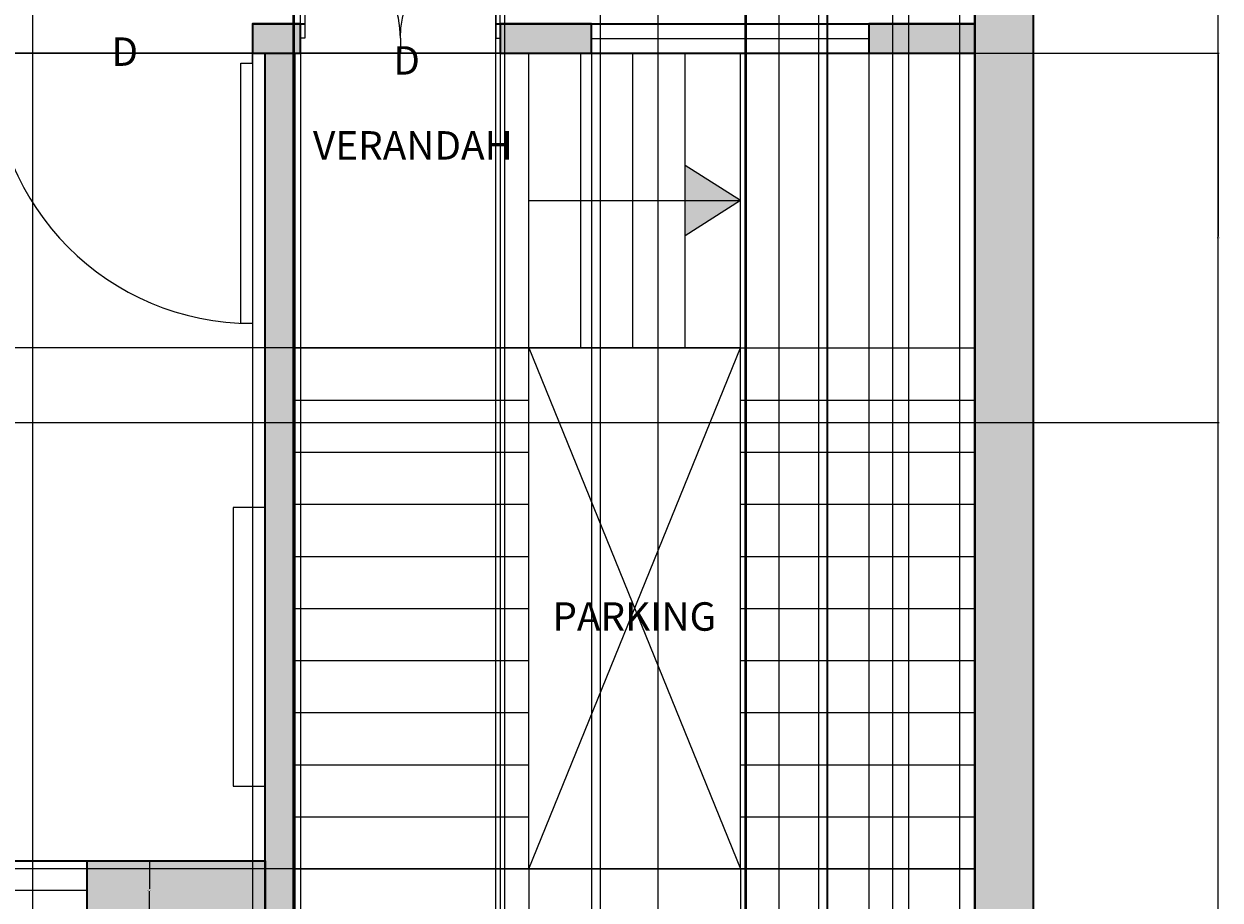
# Model space of a CAD drawing. Units: inches. Extents: x 2035 to 2384, y 1427 to 2020.
# Tile 3 of 7: x 2200 to 2383, y 1551 to 1685. Entities that reach past the tile are written whole.
import ezdxf

# ---------------------------------------------------------------- set-up
doc = ezdxf.new("R2010")
doc.units = ezdxf.units.IN
for name, color, linetype, lineweight in [('A-ANNO-DIMS', 2, 'Continuous', 18), ('A-ANNO-IDEN', 201, 'Continuous', 18), ('A-ANNO-SYMB', 201, 'Continuous', 18), ('A-AREA-IDEN', 201, 'Continuous', 18), ('A-FLOR-STRS', 8, 'Continuous', 18), ('A-WALL-PATT', 140, 'Continuous', 13), ('C-PROP', 7, 'Continuous', 25), ('DOOR', 52, 'Continuous', 25), ('FUR', 71, 'Continuous', 18), ('WALL', 140, 'Continuous', 35), ('WIN', 230, 'Continuous', 18)]:
    doc.layers.add(name, color=color, linetype=linetype, lineweight=lineweight)
doc.styles.get("Standard").update_dxf_attribs({"font": 'arial.ttf'})
doc.dimstyles.get("Standard").update_dxf_attribs({"dimtxt": 0.18, "dimasz": 0.18, "dimexe": 0.18, "dimexo": 0.0625, "dimgap": 0.09, "dimtad": 0, "dimtih": 1, "dimtoh": 1, "dimdec": 4, "dimzin": 0, "dimdsep": 46, "dimtxsty": 'Standard', "dimcen": 0.09, "dimadec": 0, "dimazin": 0, "dimtfac": 1, "dimtdec": 4, "dimtofl": 0, "dimtmove": 0, "dimatfit": 3, "dimfxl": 1, "dimtolj": 1, "dimtzin": 0, "dimarcsym": 0})

# ---------------------------------------------------------------- blocks, each defined once
blk = doc.blocks.new('*U2')
for p, q in [((0, 0), (0, -6)), ((40, 0), (40, -6))]:
    blk.add_line(p, q)
blk.add_lwpolyline([(0, 0), (0, 40), (1.75, 40), (1.75, 0)], close=True)
blk.add_arc((0, 0), 40, 0, 90)
blk = doc.blocks.new('WIN-BEDROOM')
blk.add_line((0, 4.5), (63.76, 4.5))
blk.add_lwpolyline([(0, 9), (63.76, 9), (63.76, 0), (0, 0)], close=True)
blk = doc.blocks.new('*D15')
at = {"layer": 'A-ANNO-DIMS', "color": 0, "lineweight": -2, "transparency": 16777216}
for p, q in [((2209.44, 1556.88), (2219.12, 1556.88)), ((2218.94, 1556.7), (2218.94, 1552.56)), ((2218.94, 1548.06), (2218.94, 1552.2)), ((2209.44, 1547.88), (2219.12, 1547.88))]:
    blk.add_line(p, q, dxfattribs=at)
at = {"layer": 'A-ANNO-DIMS', "color": 0, "lineweight": 100, "transparency": 16777216}
for points in [[(2218.91, 1556.7), (2218.97, 1556.7), (2218.94, 1556.88)], [(2218.91, 1548.06), (2218.97, 1548.06), (2218.94, 1547.88)]]:
    blk.add_solid(points, dxfattribs=at)
at = {"layer": 'Defpoints', "color": 0, "lineweight": 100, "transparency": 16777216}
for p in [(2209.38, 1556.88), (2218.94, 1556.88), (2209.38, 1547.88)]:
    blk.add_point(p, dxfattribs=at)
at = {"layer": 'A-ANNO-DIMS', "color": 0, "transparency": 16777216, "insert": (2218.94, 1552.38), "char_height": 0.18, "attachment_point": 5}
blk.add_mtext('\\A1;9 TYP.', dxfattribs=at)
blk = doc.blocks.new('*D23')
at = {"layer": 'A-ANNO-DIMS', "color": 0, "lineweight": -2, "transparency": 16777216}
for p, q in [((2354.82, 1981.38), (2383.33, 1981.38)), ((2383.15, 1981.2), (2383.15, 1741.56)), ((2383.15, 1501.56), (2383.15, 1741.2)), ((2354.82, 1501.38), (2383.33, 1501.38))]:
    blk.add_line(p, q, dxfattribs=at)
at = {"layer": 'A-ANNO-DIMS', "color": 0, "lineweight": 100, "transparency": 16777216}
for points in [[(2383.12, 1981.2), (2383.18, 1981.2), (2383.15, 1981.38)], [(2383.12, 1501.56), (2383.18, 1501.56), (2383.15, 1501.38)]]:
    blk.add_solid(points, dxfattribs=at)
at = {"layer": 'Defpoints', "color": 0, "lineweight": 100, "transparency": 16777216}
for p in [(2354.75, 1981.38), (2383.15, 1981.38), (2354.75, 1501.38)]:
    blk.add_point(p, dxfattribs=at)
at = {"layer": 'A-ANNO-DIMS', "color": 0, "transparency": 16777216, "insert": (2383.15, 1741.38), "char_height": 0.18, "attachment_point": 5}
blk.add_mtext('\\A1;480', dxfattribs=at)
blk = doc.blocks.new('*D25')
at = {"layer": 'A-ANNO-DIMS', "color": 0, "lineweight": -2, "transparency": 16777216}
for p, q in [((2241.25, 1503.69), (2241.25, 2009.96)), ((2241.43, 2009.78), (2256.26, 2009.78)), ((2272.01, 2009.78), (2257.18, 2009.78)), ((2272.19, 1503.69), (2272.19, 2009.96))]:
    blk.add_line(p, q, dxfattribs=at)
at = {"layer": 'A-ANNO-DIMS', "color": 0, "lineweight": 100, "transparency": 16777216}
for points in [[(2241.43, 2009.81), (2241.43, 2009.75), (2241.25, 2009.78)], [(2272.01, 2009.81), (2272.01, 2009.75), (2272.19, 2009.78)]]:
    blk.add_solid(points, dxfattribs=at)
at = {"layer": 'Defpoints', "color": 0, "lineweight": 100, "transparency": 16777216}
for p in [(2272.19, 2009.78), (2241.25, 1503.63), (2272.19, 1503.63)]:
    blk.add_point(p, dxfattribs=at)
at = {"layer": 'A-ANNO-DIMS', "color": 0, "transparency": 16777216, "insert": (2256.72, 2009.78), "char_height": 0.18, "attachment_point": 5}
blk.add_mtext('\\A1;30.935', dxfattribs=at)
blk = doc.blocks.new('*D26')
at = {"layer": 'A-ANNO-DIMS', "color": 0, "lineweight": -2, "transparency": 16777216}
for p, q in [((2272.19, 1506.56), (2272.19, 2009.96)), ((2272.37, 2009.78), (2297.26, 2009.78)), ((2322.93, 2009.78), (2298.04, 2009.78)), ((2323.11, 1506.56), (2323.11, 2009.96))]:
    blk.add_line(p, q, dxfattribs=at)
at = {"layer": 'A-ANNO-DIMS', "color": 0, "lineweight": 100, "transparency": 16777216}
for points in [[(2272.37, 2009.81), (2272.37, 2009.75), (2272.19, 2009.78)], [(2322.93, 2009.81), (2322.93, 2009.75), (2323.11, 2009.78)]]:
    blk.add_solid(points, dxfattribs=at)
at = {"layer": 'Defpoints', "color": 0, "lineweight": 100, "transparency": 16777216}
for p in [(2323.11, 2009.78), (2272.19, 1506.5), (2323.11, 1506.5)]:
    blk.add_point(p, dxfattribs=at)
at = {"layer": 'A-ANNO-DIMS', "color": 0, "transparency": 16777216, "insert": (2297.65, 2009.78), "char_height": 0.18, "attachment_point": 5}
blk.add_mtext('\\A1;50.92', dxfattribs=at)
blk = doc.blocks.new('*D28')
at = {"layer": 'A-ANNO-DIMS', "color": 0, "lineweight": -2, "transparency": 16777216}
for p, q in [((2345.69, 1555.63), (2035.17, 1555.63)), ((2035.35, 1555.45), (2035.35, 1531.25)), ((2035.35, 1506.68), (2035.35, 1530.88)), ((2323.05, 1506.5), (2035.17, 1506.5))]:
    blk.add_line(p, q, dxfattribs=at)
at = {"layer": 'A-ANNO-DIMS', "color": 0, "lineweight": 100, "transparency": 16777216}
for points in [[(2035.32, 1555.45), (2035.38, 1555.45), (2035.35, 1555.63)], [(2035.32, 1506.68), (2035.38, 1506.68), (2035.35, 1506.5)]]:
    blk.add_solid(points, dxfattribs=at)
at = {"layer": 'Defpoints', "color": 0, "lineweight": 100, "transparency": 16777216}
for p in [(2035.35, 1555.63), (2345.75, 1555.63), (2323.11, 1506.5)]:
    blk.add_point(p, dxfattribs=at)
at = {"layer": 'A-ANNO-DIMS', "color": 0, "transparency": 16777216, "insert": (2035.35, 1531.06), "char_height": 0.18, "attachment_point": 5}
blk.add_mtext('\\A1;49.14', dxfattribs=at)
blk = doc.blocks.new('*D29')
at = {"layer": 'A-ANNO-DIMS', "color": 0, "lineweight": -2, "transparency": 16777216}
for p, q in [((2309.69, 1635.63), (2035.17, 1635.63)), ((2035.35, 1635.45), (2035.35, 1595.81)), ((2035.35, 1555.81), (2035.35, 1595.45)), ((2309.69, 1555.63), (2035.17, 1555.63))]:
    blk.add_line(p, q, dxfattribs=at)
at = {"layer": 'A-ANNO-DIMS', "color": 0, "lineweight": 100, "transparency": 16777216}
for points in [[(2035.32, 1635.45), (2035.38, 1635.45), (2035.35, 1635.63)], [(2035.32, 1555.81), (2035.38, 1555.81), (2035.35, 1555.63)]]:
    blk.add_solid(points, dxfattribs=at)
at = {"layer": 'Defpoints', "color": 0, "lineweight": 100, "transparency": 16777216}
for p in [(2035.35, 1635.63), (2309.75, 1635.63), (2309.75, 1555.63)]:
    blk.add_point(p, dxfattribs=at)
at = {"layer": 'A-ANNO-DIMS', "color": 0, "transparency": 16777216, "insert": (2035.35, 1595.63), "char_height": 0.18, "attachment_point": 5}
blk.add_mtext('\\A1;80', dxfattribs=at)
blk = doc.blocks.new('*D30')
at = {"layer": 'A-ANNO-DIMS', "color": 0, "lineweight": -2, "transparency": 16777216}
for p, q in [((2309.69, 1680.88), (2035.17, 1680.88)), ((2035.35, 1680.7), (2035.35, 1658.44)), ((2035.35, 1635.81), (2035.35, 1658.07)), ((2309.69, 1635.63), (2035.17, 1635.63))]:
    blk.add_line(p, q, dxfattribs=at)
at = {"layer": 'A-ANNO-DIMS', "color": 0, "lineweight": 100, "transparency": 16777216}
for points in [[(2035.32, 1680.7), (2035.38, 1680.7), (2035.35, 1680.88)], [(2035.32, 1635.81), (2035.38, 1635.81), (2035.35, 1635.63)]]:
    blk.add_solid(points, dxfattribs=at)
at = {"layer": 'Defpoints', "color": 0, "lineweight": 100, "transparency": 16777216}
for p in [(2035.35, 1680.88), (2309.75, 1680.88), (2309.75, 1635.63)]:
    blk.add_point(p, dxfattribs=at)
at = {"layer": 'A-ANNO-DIMS', "color": 0, "transparency": 16777216, "insert": (2035.35, 1658.26), "char_height": 0.18, "attachment_point": 5}
blk.add_mtext('\\A1;45.25', dxfattribs=at)
blk = doc.blocks.new('*D31')
at = {"layer": 'A-ANNO-DIMS', "color": 0, "lineweight": -2, "transparency": 16777216}
for p, q in [((2241.25, 1555.57), (2241.25, 1427.17)), ((2277.25, 1555.57), (2277.25, 1427.17)), ((2241.43, 1427.35), (2259.03, 1427.35)), ((2277.07, 1427.35), (2259.47, 1427.35))]:
    blk.add_line(p, q, dxfattribs=at)
at = {"layer": 'A-ANNO-DIMS', "color": 0, "lineweight": 100, "transparency": 16777216}
for points in [[(2241.43, 1427.38), (2241.43, 1427.32), (2241.25, 1427.35)], [(2277.07, 1427.38), (2277.07, 1427.32), (2277.25, 1427.35)]]:
    blk.add_solid(points, dxfattribs=at)
at = {"layer": 'Defpoints', "color": 0, "lineweight": 100, "transparency": 16777216}
for p in [(2241.25, 1555.63), (2277.25, 1555.63), (2277.25, 1427.35)]:
    blk.add_point(p, dxfattribs=at)
at = {"layer": 'A-ANNO-DIMS', "color": 0, "transparency": 16777216, "insert": (2259.25, 1427.35), "char_height": 0.18, "attachment_point": 5}
blk.add_mtext('\\A1;36', dxfattribs=at)
blk = doc.blocks.new('*D32')
at = {"layer": 'A-ANNO-DIMS', "color": 0, "lineweight": -2, "transparency": 16777216}
for p, q in [((2277.25, 1555.57), (2277.25, 1427.17)), ((2309.75, 1555.57), (2309.75, 1427.17)), ((2277.43, 1427.35), (2293.18, 1427.35)), ((2309.57, 1427.35), (2293.83, 1427.35))]:
    blk.add_line(p, q, dxfattribs=at)
at = {"layer": 'A-ANNO-DIMS', "color": 0, "lineweight": 100, "transparency": 16777216}
for points in [[(2277.43, 1427.38), (2277.43, 1427.32), (2277.25, 1427.35)], [(2309.57, 1427.38), (2309.57, 1427.32), (2309.75, 1427.35)]]:
    blk.add_solid(points, dxfattribs=at)
at = {"layer": 'Defpoints', "color": 0, "lineweight": 100, "transparency": 16777216}
for p in [(2277.25, 1555.63), (2309.75, 1555.63), (2309.75, 1427.35)]:
    blk.add_point(p, dxfattribs=at)
at = {"layer": 'A-ANNO-DIMS', "color": 0, "transparency": 16777216, "insert": (2293.5, 1427.35), "char_height": 0.18, "attachment_point": 5}
blk.add_mtext('\\A1;32.5', dxfattribs=at)
blk = doc.blocks.new('*D34')
at = {"layer": 'A-ANNO-DIMS', "color": 0, "lineweight": -2, "transparency": 16777216}
for p, q in [((2194.77, 1680.82), (2194.77, 1427.17)), ((2234.77, 1680.82), (2234.77, 1427.17)), ((2194.95, 1427.35), (2214.55, 1427.35)), ((2234.59, 1427.35), (2214.99, 1427.35))]:
    blk.add_line(p, q, dxfattribs=at)
at = {"layer": 'A-ANNO-DIMS', "color": 0, "lineweight": 100, "transparency": 16777216}
for points in [[(2194.95, 1427.38), (2194.95, 1427.32), (2194.77, 1427.35)], [(2234.59, 1427.38), (2234.59, 1427.32), (2234.77, 1427.35)]]:
    blk.add_solid(points, dxfattribs=at)
at = {"layer": 'Defpoints', "color": 0, "lineweight": 100, "transparency": 16777216}
for p in [(2194.77, 1680.88), (2234.77, 1680.88), (2234.77, 1427.35)]:
    blk.add_point(p, dxfattribs=at)
at = {"layer": 'A-ANNO-DIMS', "color": 0, "transparency": 16777216, "insert": (2214.77, 1427.35), "char_height": 0.18, "attachment_point": 5}
blk.add_mtext('\\A1;40', dxfattribs=at)
blk = doc.blocks.new('*D35')
at = {"layer": 'A-ANNO-DIMS', "color": 0, "lineweight": -2, "transparency": 16777216}
for p, q in [((2242.18, 1680.82), (2242.18, 1427.17)), ((2272.85, 1680.82), (2272.85, 1427.17)), ((2242.36, 1427.35), (2257.05, 1427.35)), ((2272.67, 1427.35), (2257.98, 1427.35))]:
    blk.add_line(p, q, dxfattribs=at)
at = {"layer": 'A-ANNO-DIMS', "color": 0, "lineweight": 100, "transparency": 16777216}
for points in [[(2242.36, 1427.38), (2242.36, 1427.32), (2242.18, 1427.35)], [(2272.67, 1427.38), (2272.67, 1427.32), (2272.85, 1427.35)]]:
    blk.add_solid(points, dxfattribs=at)
at = {"layer": 'Defpoints', "color": 0, "lineweight": 100, "transparency": 16777216}
for p in [(2242.18, 1680.88), (2272.85, 1680.88), (2272.85, 1427.35)]:
    blk.add_point(p, dxfattribs=at)
at = {"layer": 'A-ANNO-DIMS', "color": 0, "transparency": 16777216, "insert": (2257.52, 1427.35), "char_height": 0.18, "attachment_point": 5}
blk.add_mtext('\\A1;30.676', dxfattribs=at)
blk = doc.blocks.new('*D36')
at = {"layer": 'A-ANNO-DIMS', "color": 0, "lineweight": -2, "transparency": 16777216}
for p, q in [((2286.88, 1680.82), (2286.88, 1427.17)), ((2329.51, 1680.82), (2329.51, 1427.17)), ((2287.06, 1427.35), (2307.8, 1427.35)), ((2329.33, 1427.35), (2308.59, 1427.35))]:
    blk.add_line(p, q, dxfattribs=at)
at = {"layer": 'A-ANNO-DIMS', "color": 0, "lineweight": 100, "transparency": 16777216}
for points in [[(2287.06, 1427.38), (2287.06, 1427.32), (2286.88, 1427.35)], [(2329.33, 1427.38), (2329.33, 1427.32), (2329.51, 1427.35)]]:
    blk.add_solid(points, dxfattribs=at)
at = {"layer": 'Defpoints', "color": 0, "lineweight": 100, "transparency": 16777216}
for p in [(2286.88, 1680.88), (2329.51, 1680.88), (2329.51, 1427.35)]:
    blk.add_point(p, dxfattribs=at)
at = {"layer": 'A-ANNO-DIMS', "color": 0, "transparency": 16777216, "insert": (2308.2, 1427.35), "char_height": 0.18, "attachment_point": 5}
blk.add_mtext('\\A1;42.63', dxfattribs=at)
blk = doc.blocks.new('*D40')
at = {"layer": 'A-ANNO-DIMS', "color": 0, "lineweight": -2, "transparency": 16777216}
for p, q in [((2201.01, 1835.82), (2201.01, 1427.17)), ((2241.01, 1835.82), (2241.01, 1427.17)), ((2201.19, 1427.35), (2220.79, 1427.35)), ((2240.83, 1427.35), (2221.24, 1427.35))]:
    blk.add_line(p, q, dxfattribs=at)
at = {"layer": 'A-ANNO-DIMS', "color": 0, "lineweight": 100, "transparency": 16777216}
for points in [[(2201.19, 1427.38), (2201.19, 1427.32), (2201.01, 1427.35)], [(2240.83, 1427.38), (2240.83, 1427.32), (2241.01, 1427.35)]]:
    blk.add_solid(points, dxfattribs=at)
at = {"layer": 'Defpoints', "color": 0, "lineweight": 100, "transparency": 16777216}
for p in [(2201.01, 1835.88), (2241.01, 1835.88), (2241.01, 1427.35)]:
    blk.add_point(p, dxfattribs=at)
at = {"layer": 'A-ANNO-DIMS', "color": 0, "transparency": 16777216, "insert": (2221.01, 1427.35), "char_height": 0.18, "attachment_point": 5}
blk.add_mtext('\\A1;40', dxfattribs=at)
blk = doc.blocks.new('*D41')
at = {"layer": 'A-ANNO-DIMS', "color": 0, "lineweight": -2, "transparency": 16777216}
for p, q in [((2273.51, 1840.32), (2273.51, 1427.17)), ((2310.46, 1840.32), (2310.46, 1427.17)), ((2273.69, 1427.35), (2291.59, 1427.35)), ((2310.28, 1427.35), (2292.38, 1427.35))]:
    blk.add_line(p, q, dxfattribs=at)
at = {"layer": 'A-ANNO-DIMS', "color": 0, "lineweight": 100, "transparency": 16777216}
for points in [[(2273.69, 1427.38), (2273.69, 1427.32), (2273.51, 1427.35)], [(2310.28, 1427.38), (2310.28, 1427.32), (2310.46, 1427.35)]]:
    blk.add_solid(points, dxfattribs=at)
at = {"layer": 'Defpoints', "color": 0, "lineweight": 100, "transparency": 16777216}
for p in [(2273.51, 1840.38), (2310.46, 1840.38), (2310.46, 1427.35)]:
    blk.add_point(p, dxfattribs=at)
at = {"layer": 'A-ANNO-DIMS', "color": 0, "transparency": 16777216, "insert": (2291.98, 1427.35), "char_height": 0.18, "attachment_point": 5}
blk.add_mtext('\\A1;36.95', dxfattribs=at)
blk = doc.blocks.new('*D42')
at = {"layer": 'A-ANNO-DIMS', "color": 0, "lineweight": -2, "transparency": 16777216}
for p, q in [((2297.05, 1925.82), (2297.05, 1427.17)), ((2333.11, 1925.82), (2333.11, 1427.17)), ((2297.23, 1427.35), (2314.69, 1427.35)), ((2332.93, 1427.35), (2315.47, 1427.35))]:
    blk.add_line(p, q, dxfattribs=at)
at = {"layer": 'A-ANNO-DIMS', "color": 0, "lineweight": 100, "transparency": 16777216}
for points in [[(2297.23, 1427.38), (2297.23, 1427.32), (2297.05, 1427.35)], [(2332.93, 1427.38), (2332.93, 1427.32), (2333.11, 1427.35)]]:
    blk.add_solid(points, dxfattribs=at)
at = {"layer": 'Defpoints', "color": 0, "lineweight": 100, "transparency": 16777216}
for p in [(2297.05, 1925.88), (2333.11, 1925.88), (2333.11, 1427.35)]:
    blk.add_point(p, dxfattribs=at)
at = {"layer": 'A-ANNO-DIMS', "color": 0, "transparency": 16777216, "insert": (2315.08, 1427.35), "char_height": 0.18, "attachment_point": 5}
blk.add_mtext('\\A1;36.06', dxfattribs=at)
blk = doc.blocks.new('*D45')
at = {"layer": 'A-ANNO-DIMS', "color": 0, "lineweight": -2, "transparency": 16777216}
for p, q in [((2321.75, 1840.32), (2321.75, 1427.17)), ((2345.75, 1840.32), (2345.75, 1427.17)), ((2321.93, 1427.35), (2333.53, 1427.35)), ((2345.57, 1427.35), (2333.97, 1427.35))]:
    blk.add_line(p, q, dxfattribs=at)
at = {"layer": 'A-ANNO-DIMS', "color": 0, "lineweight": 100, "transparency": 16777216}
for points in [[(2321.93, 1427.38), (2321.93, 1427.32), (2321.75, 1427.35)], [(2345.57, 1427.38), (2345.57, 1427.32), (2345.75, 1427.35)]]:
    blk.add_solid(points, dxfattribs=at)
at = {"layer": 'Defpoints', "color": 0, "lineweight": 100, "transparency": 16777216}
for p in [(2321.75, 1840.38), (2345.75, 1840.38), (2345.75, 1427.35)]:
    blk.add_point(p, dxfattribs=at)
at = {"layer": 'A-ANNO-DIMS', "color": 0, "transparency": 16777216, "insert": (2333.75, 1427.35), "char_height": 0.18, "attachment_point": 5}
blk.add_mtext('\\A1;24', dxfattribs=at)
blk = doc.blocks.new('*D46')
at = {"layer": 'A-ANNO-DIMS', "color": 0, "lineweight": -2, "transparency": 16777216}
for p, q in [((2288.19, 1905.68), (2288.19, 1427.17)), ((2315.66, 1905.68), (2315.66, 1427.17)), ((2288.37, 1427.35), (2301.53, 1427.35)), ((2315.48, 1427.35), (2302.32, 1427.35))]:
    blk.add_line(p, q, dxfattribs=at)
at = {"layer": 'A-ANNO-DIMS', "color": 0, "lineweight": 100, "transparency": 16777216}
for points in [[(2288.37, 1427.38), (2288.37, 1427.32), (2288.19, 1427.35)], [(2315.48, 1427.38), (2315.48, 1427.32), (2315.66, 1427.35)]]:
    blk.add_solid(points, dxfattribs=at)
at = {"layer": 'Defpoints', "color": 0, "lineweight": 100, "transparency": 16777216}
for p in [(2288.19, 1905.75), (2315.66, 1905.75), (2315.66, 1427.35)]:
    blk.add_point(p, dxfattribs=at)
at = {"layer": 'A-ANNO-DIMS', "color": 0, "transparency": 16777216, "insert": (2301.92, 1427.35), "char_height": 0.18, "attachment_point": 5}
blk.add_mtext('\\A1;27.47', dxfattribs=at)
blk = doc.blocks.new('*D48')
at = {"layer": 'A-ANNO-DIMS', "color": 0, "lineweight": -2, "transparency": 16777216}
for p, q in [((2323.12, 1858.3), (2323.12, 1427.17)), ((2343.42, 1858.3), (2343.42, 1427.17)), ((2323.3, 1427.35), (2332.81, 1427.35)), ((2343.24, 1427.35), (2333.74, 1427.35))]:
    blk.add_line(p, q, dxfattribs=at)
at = {"layer": 'A-ANNO-DIMS', "color": 0, "lineweight": 100, "transparency": 16777216}
for points in [[(2323.3, 1427.38), (2323.3, 1427.32), (2323.12, 1427.35)], [(2343.24, 1427.38), (2343.24, 1427.32), (2343.42, 1427.35)]]:
    blk.add_solid(points, dxfattribs=at)
at = {"layer": 'Defpoints', "color": 0, "lineweight": 100, "transparency": 16777216}
for p in [(2323.12, 1858.36), (2343.42, 1858.36), (2343.42, 1427.35)]:
    blk.add_point(p, dxfattribs=at)
at = {"layer": 'A-ANNO-DIMS', "color": 0, "transparency": 16777216, "insert": (2333.27, 1427.35), "char_height": 0.18, "attachment_point": 5}
blk.add_mtext('\\A1;20.302', dxfattribs=at)
blk = doc.blocks.new('*D57')
at = {"layer": 'A-ANNO-DIMS', "color": 0, "lineweight": -2, "transparency": 16777216}
for p, q in [((2310.65, 1726.38), (2310.65, 1427.17)), ((2335.58, 1723.97), (2335.58, 1427.17)), ((2310.83, 1427.35), (2322.65, 1427.35)), ((2335.4, 1427.35), (2323.58, 1427.35))]:
    blk.add_line(p, q, dxfattribs=at)
at = {"layer": 'A-ANNO-DIMS', "color": 0, "lineweight": 100, "transparency": 16777216}
for points in [[(2310.83, 1427.38), (2310.83, 1427.32), (2310.65, 1427.35)], [(2335.4, 1427.38), (2335.4, 1427.32), (2335.58, 1427.35)]]:
    blk.add_solid(points, dxfattribs=at)
at = {"layer": 'Defpoints', "color": 0, "lineweight": 100, "transparency": 16777216}
for p in [(2310.65, 1726.45), (2335.58, 1724.03), (2335.58, 1427.35)]:
    blk.add_point(p, dxfattribs=at)
at = {"layer": 'A-ANNO-DIMS', "color": 0, "transparency": 16777216, "insert": (2323.12, 1427.35), "char_height": 0.18, "attachment_point": 5}
blk.add_mtext('\\A1;24.924', dxfattribs=at)
blk = doc.blocks.new('*D63')
at = {"layer": 'A-ANNO-DIMS', "color": 0, "lineweight": -2, "transparency": 16777216}
for p, q in [((2144.84, 1680.88), (2383.33, 1680.88)), ((2383.15, 1680.7), (2383.15, 1652.72)), ((2383.15, 1624.38), (2383.15, 1652.36)), ((2144.84, 1624.2), (2383.33, 1624.2))]:
    blk.add_line(p, q, dxfattribs=at)
at = {"layer": 'A-ANNO-DIMS', "color": 0, "lineweight": 100, "transparency": 16777216}
for points in [[(2383.12, 1680.7), (2383.18, 1680.7), (2383.15, 1680.88)], [(2383.12, 1624.38), (2383.18, 1624.38), (2383.15, 1624.2)]]:
    blk.add_solid(points, dxfattribs=at)
at = {"layer": 'Defpoints', "color": 0, "lineweight": 100, "transparency": 16777216}
for p in [(2144.78, 1680.88), (2383.15, 1680.88), (2144.78, 1624.2)]:
    blk.add_point(p, dxfattribs=at)
at = {"layer": 'A-ANNO-DIMS', "color": 0, "transparency": 16777216, "insert": (2383.15, 1652.54), "char_height": 0.18, "attachment_point": 5}
blk.add_mtext('\\A1;56.68', dxfattribs=at)
blk = doc.blocks.new('*D64')
at = {"layer": 'A-ANNO-DIMS', "color": 0, "lineweight": -2, "transparency": 16777216}
for p, q in [((2335.58, 1723.97), (2335.58, 1427.17)), ((2345.75, 1685.32), (2345.75, 1427.17)), ((2335.76, 1427.35), (2340.21, 1427.35)), ((2345.57, 1427.35), (2341.12, 1427.35))]:
    blk.add_line(p, q, dxfattribs=at)
at = {"layer": 'A-ANNO-DIMS', "color": 0, "lineweight": 100, "transparency": 16777216}
for points in [[(2335.76, 1427.38), (2335.76, 1427.32), (2335.58, 1427.35)], [(2345.57, 1427.38), (2345.57, 1427.32), (2345.75, 1427.35)]]:
    blk.add_solid(points, dxfattribs=at)
at = {"layer": 'Defpoints', "color": 0, "lineweight": 100, "transparency": 16777216}
for p in [(2335.58, 1724.03), (2345.75, 1685.38), (2345.75, 1427.35)]:
    blk.add_point(p, dxfattribs=at)
at = {"layer": 'A-ANNO-DIMS', "color": 0, "transparency": 16777216, "insert": (2340.67, 1427.35), "char_height": 0.18, "attachment_point": 5}
blk.add_mtext('\\A1;10.174', dxfattribs=at)
blk = doc.blocks.new('*D67')
at = {"layer": 'A-ANNO-DIMS', "color": 0, "lineweight": -2, "transparency": 16777216}
for p, q in [((2272.85, 1680.82), (2272.85, 1427.17)), ((2286.88, 1680.82), (2286.88, 1427.17)), ((2273.03, 1427.35), (2279.41, 1427.35)), ((2286.7, 1427.35), (2280.32, 1427.35))]:
    blk.add_line(p, q, dxfattribs=at)
at = {"layer": 'A-ANNO-DIMS', "color": 0, "lineweight": 100, "transparency": 16777216}
for points in [[(2273.03, 1427.38), (2273.03, 1427.32), (2272.85, 1427.35)], [(2286.7, 1427.38), (2286.7, 1427.32), (2286.88, 1427.35)]]:
    blk.add_solid(points, dxfattribs=at)
at = {"layer": 'Defpoints', "color": 0, "lineweight": 100, "transparency": 16777216}
for p in [(2272.85, 1680.88), (2286.88, 1680.88), (2286.88, 1427.35)]:
    blk.add_point(p, dxfattribs=at)
at = {"layer": 'A-ANNO-DIMS', "color": 0, "transparency": 16777216, "insert": (2279.87, 1427.35), "char_height": 0.18, "attachment_point": 5}
blk.add_mtext('\\A1;14.025', dxfattribs=at)

msp = doc.modelspace()

# ---------------------------------------------------------------- hatches: boundary and pattern name
at = {"layer": 'A-ANNO-SYMB'}
h = msp.add_hatch(color=256, dxfattribs=at)
h.dxf.hatch_style = 1
h.paths.add_polyline_path([(2309.7529, 1658.2566), (2301.2529, 1658.2566), (2301.2529, 1652.8522)])
h.paths.add_polyline_path([(2301.2529, 1663.6609), (2301.2529, 1658.2566), (2309.7529, 1658.2566)])
at = {"layer": 'A-WALL-PATT'}
h = msp.add_hatch(color=256, dxfattribs=at)
h.dxf.hatch_style = 1
h.paths.add_polyline_path([(2145.6215, 1981.3816), (2123.7529, 1981.3816), (2123.7529, 1972.3816), (2145.6215, 1972.3816)])
h.paths.add_polyline_path([(2354.7529, 1981.3816), (2209.3767, 1981.3816), (2209.3767, 1972.3816), (2354.7529, 1972.3816)])
h.paths.add_polyline_path([(2123.7529, 1981.3816), (2114.7529, 1981.3816), (2114.7529, 1505.8816), (2123.7529, 1505.8816)])
h.paths.add_polyline_path([(2248.2529, 1928.1316), (2243.7529, 1928.1316), (2243.7529, 1840.3816), (2248.2529, 1840.3816)])
h.paths.add_polyline_path([(2297.0514, 1930.3816), (2284.6994, 1930.3816), (2284.6994, 1925.8816), (2297.0514, 1925.8816)])
h.paths.add_polyline_path([(2345.7529, 1930.3816), (2333.1098, 1930.3816), (2333.1098, 1925.8816), (2345.7529, 1925.8816)])
h.paths.add_polyline_path([(2354.7529, 1972.3816), (2345.7529, 1972.3816), (2345.7529, 1501.3816), (2354.7529, 1501.3816)])
h.paths.add_polyline_path([(2188.2529, 1835.8816), (2183.7529, 1835.8816), (2183.7529, 1831.3677), (2184.207, 1831.3677), (2188.2529, 1831.3677)])
h.paths.add_polyline_path([(2188.2529, 1804.3949), (2184.207, 1804.3949), (2183.7529, 1804.3949), (2183.7529, 1685.3816), (2188.2529, 1685.3816)])
h.paths.add_polyline_path([(2273.5087, 1840.3816), (2241.0146, 1840.3816), (2241.0146, 1835.8816), (2273.5087, 1835.8816)])
h.paths.add_polyline_path([(2345.7529, 1840.3816), (2310.4577, 1840.3816), (2310.4577, 1835.8816), (2345.7529, 1835.8816)])
h.paths.add_polyline_path([(2161.9064, 1524.4315), (2196.2972, 1524.4315), (2196.2972, 1533.4306), (2161.9064, 1533.4306)], flags=9)
h.paths.add_polyline_path([(2279.3058, 1589.7515), (2308.9483, 1589.7515), (2308.9483, 1598.7506), (2279.3058, 1598.7506)], flags=9)
h.paths.add_polyline_path([(2242.9684, 1662.1655), (2279.0513, 1662.1655), (2279.0513, 1671.1647), (2242.9684, 1671.1647)], flags=9)
h.paths.add_polyline_path([(2154.6483, 1622.8242), (2195.1309, 1622.8242), (2195.1309, 1639.1195), (2154.6483, 1639.1195)], flags=9)
h.paths.add_polyline_path([(2138.8708, 1715.378), (2162.5199, 1715.378), (2162.5199, 1731.6734), (2138.8708, 1731.6734)], flags=9)
h.paths.add_polyline_path([(2135.5598, 1791.707), (2165.1993, 1791.707), (2165.1993, 1808.0024), (2135.5598, 1808.0024)], flags=9)
h.paths.add_polyline_path([(2245.1071, 1740.4502), (2279.0303, 1740.4502), (2279.0303, 1756.7455), (2245.1071, 1756.7455)], flags=9)
h.paths.add_polyline_path([(2284.7312, 1866.5552), (2313.6916, 1866.5552), (2313.6916, 1890.2034), (2284.7312, 1890.2034)], flags=9)
h.paths.add_polyline_path([(2139.9071, 1874.6496), (2173.8303, 1874.6496), (2173.8303, 1890.9449), (2139.9071, 1890.9449)], flags=9)
h = msp.add_hatch(color=256, dxfattribs=at)
h.dxf.hatch_style = 1
h.paths.add_polyline_path([(2236.7529, 1556.8816), (2209.3767, 1556.8816), (2209.3767, 1547.8816), (2236.7529, 1547.8816)])
h.paths.add_polyline_path([(2241.2529, 1680.8816), (2236.7529, 1680.8816), (2236.7529, 1547.8816), (2241.2529, 1547.8816)])
h.paths.add_polyline_path([(2241.2529, 1505.8816), (2114.7529, 1505.8816), (2114.7529, 1501.3816), (2241.2529, 1501.3816)])
h.paths.add_polyline_path([(2242.179, 1683.1823), (2242.179, 1685.3816), (2234.769, 1685.3816), (2234.769, 1680.8816), (2242.179, 1680.8816)])
h.paths.add_polyline_path([(2286.8795, 1685.3816), (2272.8549, 1685.3816), (2272.8549, 1683.1823), (2272.8549, 1680.8816), (2286.8795, 1680.8816)])
h.paths.add_polyline_path([(2345.7529, 1685.3816), (2329.513, 1685.3816), (2329.513, 1680.8816), (2345.7529, 1680.8816)])
h.paths.add_polyline_path([(2279.3058, 1589.7515), (2308.9483, 1589.7515), (2308.9483, 1598.7506), (2279.3058, 1598.7506)], flags=9)
h.paths.add_polyline_path([(2242.9684, 1662.1655), (2279.0513, 1662.1655), (2279.0513, 1671.1647), (2242.9684, 1671.1647)], flags=9)
h.paths.add_polyline_path([(2154.6483, 1622.8242), (2195.1309, 1622.8242), (2195.1309, 1639.1195), (2154.6483, 1639.1195)], flags=9)
h.paths.add_polyline_path([(2138.8708, 1715.378), (2162.5199, 1715.378), (2162.5199, 1731.6734), (2138.8708, 1731.6734)], flags=9)
h.paths.add_polyline_path([(2135.5598, 1791.707), (2165.1993, 1791.707), (2165.1993, 1808.0024), (2135.5598, 1808.0024)], flags=9)
h.paths.add_polyline_path([(2245.1071, 1740.4502), (2279.0303, 1740.4502), (2279.0303, 1756.7455), (2245.1071, 1756.7455)], flags=9)
h.paths.add_polyline_path([(2284.7312, 1866.5552), (2313.6916, 1866.5552), (2313.6916, 1890.2034), (2284.7312, 1890.2034)], flags=9)
h.paths.add_polyline_path([(2284.6985, 1943.1527), (2309.7208, 1943.1527), (2309.7208, 1959.448), (2284.6985, 1959.448)], flags=9)
h.paths.add_polyline_path([(2139.9071, 1874.6496), (2173.8303, 1874.6496), (2173.8303, 1890.9449), (2139.9071, 1890.9449)], flags=9)
h = msp.add_hatch(color=256, dxfattribs=at)
h.dxf.hatch_style = 1
h.paths.add_polyline_path([(2201.0146, 1840.3816), (2123.7529, 1840.3816), (2123.7529, 1835.8816), (2201.0146, 1835.8816)])
h.paths.add_polyline_path([(2136.2543, 1763.8816), (2123.7529, 1763.8816), (2123.7529, 1759.3816), (2136.2543, 1759.3816)])
h.paths.add_polyline_path([(2183.7529, 1763.8816), (2169.7769, 1763.8816), (2169.7769, 1759.3816), (2183.7529, 1759.3816)])
h.paths.add_polyline_path([(2152.8338, 1685.1369), (2152.8338, 1685.3816), (2123.7529, 1685.3816), (2123.7529, 1680.8816), (2152.8338, 1680.8816)])
h.paths.add_polyline_path([(2194.769, 1685.3816), (2181.2028, 1685.3816), (2181.2028, 1685.1369), (2181.2028, 1680.8816), (2194.769, 1680.8816)])
h.paths.add_polyline_path([(2145.6215, 1556.8816), (2123.7529, 1556.8816), (2123.7529, 1547.8816), (2145.6215, 1547.8816)])
h.paths.add_polyline_path([(2161.9064, 1524.4315), (2196.2972, 1524.4315), (2196.2972, 1533.4306), (2161.9064, 1533.4306)], flags=9)
h.paths.add_polyline_path([(2279.3058, 1589.7515), (2308.9483, 1589.7515), (2308.9483, 1598.7506), (2279.3058, 1598.7506)], flags=9)
h.paths.add_polyline_path([(2242.9684, 1662.1655), (2279.0513, 1662.1655), (2279.0513, 1671.1647), (2242.9684, 1671.1647)], flags=9)
h.paths.add_polyline_path([(2154.6483, 1622.8242), (2195.1309, 1622.8242), (2195.1309, 1639.1195), (2154.6483, 1639.1195)], flags=9)
h.paths.add_polyline_path([(2138.8708, 1715.378), (2162.5199, 1715.378), (2162.5199, 1731.6734), (2138.8708, 1731.6734)], flags=9)
h.paths.add_polyline_path([(2135.5598, 1791.707), (2165.1993, 1791.707), (2165.1993, 1808.0024), (2135.5598, 1808.0024)], flags=9)
h.paths.add_polyline_path([(2245.1071, 1740.4502), (2279.0303, 1740.4502), (2279.0303, 1756.7455), (2245.1071, 1756.7455)], flags=9)
h.paths.add_polyline_path([(2284.7312, 1866.5552), (2313.6916, 1866.5552), (2313.6916, 1890.2034), (2284.7312, 1890.2034)], flags=9)
h.paths.add_polyline_path([(2284.6985, 1943.1527), (2309.7208, 1943.1527), (2309.7208, 1959.448), (2284.6985, 1959.448)], flags=9)
h.paths.add_polyline_path([(2139.9071, 1874.6496), (2173.8303, 1874.6496), (2173.8303, 1890.9449), (2139.9071, 1890.9449)], flags=9)

# ---------------------------------------------------------------- linework, layer by layer
at = {"layer": 'A-ANNO-SYMB'}
for p, q in [((2309.7529, 1658.2566), (2301.2529, 1663.6609)), ((2277.2529, 1658.2566), (2309.7529, 1658.2566)), ((2309.7529, 1658.2566), (2301.2529, 1652.8522))]:
    msp.add_line(p, q, dxfattribs=at)
at = {"layer": 'A-FLOR-STRS'}
for p, q in [((2277.2529, 1635.6316), (2277.2529, 1680.8816)), ((2285.2529, 1635.6316), (2285.2529, 1680.8816)), ((2293.2529, 1635.6316), (2293.2529, 1680.8816)), ((2301.2529, 1635.6316), (2301.2529, 1680.8816)), ((2309.7529, 1635.6316), (2309.7529, 1680.8816)), ((2241.2529, 1635.6316), (2345.7529, 1635.6316)), ((2277.2529, 1555.6316), (2277.2529, 1635.6316)), ((2277.2529, 1555.6316), (2309.7529, 1635.6316)), ((2277.2529, 1635.6316), (2309.7529, 1555.6316)), ((2309.7529, 1555.6316), (2309.7529, 1635.6316)), ((2241.2529, 1627.6316), (2277.2529, 1627.6316)), ((2309.7529, 1627.6316), (2345.7529, 1627.6316)), ((2241.2529, 1619.6316), (2277.2529, 1619.6316)), ((2309.7529, 1619.6316), (2345.7529, 1619.6316)), ((2241.2529, 1611.6316), (2277.2529, 1611.6316)), ((2309.7529, 1611.6316), (2345.7529, 1611.6316)), ((2241.2529, 1603.6316), (2277.2529, 1603.6316)), ((2309.7529, 1603.6316), (2345.7529, 1603.6316)), ((2241.2529, 1595.6316), (2277.2529, 1595.6316)), ((2309.7529, 1595.6316), (2345.7529, 1595.6316)), ((2241.2529, 1587.6316), (2277.2529, 1587.6316)), ((2309.7529, 1587.6316), (2345.7529, 1587.6316)), ((2241.2529, 1579.6316), (2277.2529, 1579.6316)), ((2309.7529, 1579.6316), (2345.7529, 1579.6316)), ((2241.2529, 1571.6316), (2277.2529, 1571.6316)), ((2309.7529, 1571.6316), (2345.7529, 1571.6316)), ((2241.2529, 1563.6316), (2277.2529, 1563.6316)), ((2309.7529, 1563.6316), (2345.7529, 1563.6316)), ((2241.2529, 1555.6316), (2345.7529, 1555.6316)), ((2241.2529, 1555.6316), (2277.2529, 1555.6316)), ((2345.7529, 1555.6316), (2309.7529, 1555.6316))]:
    msp.add_line(p, q, dxfattribs=at)
at = {"layer": 'C-PROP'}
msp.add_line((2354.7529, 1981.3816), (2354.7529, 1501.3816), dxfattribs=at)
msp.add_lwpolyline([(2114.7529, 1981.3816), (2354.7529, 1981.3816), (2354.7529, 1501.3816), (2114.7529, 1501.3816)], close=True, dxfattribs=at)
at = {"layer": 'FUR'}
msp.add_lwpolyline([(2236.7529, 1611.1305), (2231.8426, 1611.1305), (2231.8426, 1568.3228), (2236.7529, 1568.3228)], close=True, dxfattribs=at)
at = {"layer": 'WALL'}
for p, q in [((2234.769, 1685.3816), (2242.85, 1685.3816)), ((2272.1838, 1685.3816), (2345.7529, 1685.3816)), ((2234.769, 1680.8816), (2242.179, 1680.8816)), ((2236.7529, 1556.8816), (2236.7529, 1680.8816)), ((2241.2529, 1552.3816), (2241.2529, 1680.8816)), ((2272.8549, 1680.8816), (2345.7529, 1680.8816)), ((2123.7529, 1556.8816), (2236.7529, 1556.8816))]:
    msp.add_line(p, q, dxfattribs=at)
msp.add_lwpolyline([(2241.2529, 1552.3816), (2241.2529, 1505.8816), (2123.7529, 1505.8816), (2123.7529, 1972.3816), (2345.7529, 1972.3816), (2345.7529, 1503.6316), (2323.1125, 1503.6316)], dxfattribs=at)
for points in [[(2345.7529, 1972.3816), (2354.7529, 1972.3816), (2354.7529, 1501.3816), (2345.7529, 1501.3816)], [(2234.769, 1680.8816), (2242.179, 1680.8816), (2242.179, 1685.3816), (2234.769, 1685.3816)], [(2272.8549, 1680.8816), (2286.8795, 1680.8816), (2286.8795, 1685.3816), (2272.8549, 1685.3816)], [(2345.7529, 1685.3816), (2329.513, 1685.3816), (2329.513, 1680.8816), (2345.7529, 1680.8816)], [(2236.7529, 1680.8816), (2241.2529, 1680.8816), (2241.2529, 1547.8816), (2236.7529, 1547.8816)], [(2209.3767, 1556.8816), (2236.7529, 1556.8816), (2236.7529, 1547.8816), (2209.3767, 1547.8816)]]:
    msp.add_lwpolyline(points, close=True, dxfattribs=at)
at = {"layer": 'WIN'}
msp.add_line((2286.8795, 1683.1316), (2329.513, 1683.1316), dxfattribs=at)
msp.add_lwpolyline([(2329.513, 1680.8816), (2286.8795, 1680.8816), (2286.8795, 1685.3816), (2329.513, 1685.3816)], close=True, dxfattribs=at)

# ---------------------------------------------------------------- block references
at = {"layer": 'DOOR', "yscale": 0.3834481157981316, "zscale": 0.3834481157981316}
for p, xscale in [((2242.179, 1683.1823), 0.3834481157981316), ((2272.8549, 1683.1823), -0.3834481157981316)]:
    msp.add_blockref('*U2', p, dxfattribs=dict(at, xscale=xscale))
at = {"layer": 'DOOR', "rotation": 180}
msp.add_blockref('*U2', (2234.769, 1679.3816), dxfattribs=at)
at = {"layer": 'WIN'}
msp.add_blockref('WIN-BEDROOM', (2145.6215, 1547.8816), dxfattribs=at)

# ---------------------------------------------------------------- texts
at = {"layer": 'A-ANNO-IDEN', "char_height": 4.367, "attachment_point": 1}
for insert in [(2213.1147, 1683.3124), (2256.421, 1681.9651)]:
    msp.add_mtext_dynamic_manual_height_columns('D', width=88.030619, gutter_width=21.835, heights=[0], dxfattribs=dict(at, insert=insert))
at = {"layer": 'A-AREA-IDEN', "char_height": 4.367, "attachment_point": 1}
for s, insert in [('VERANDAH', (2244.087, 1668.9171)), ('PARKING', (2280.8682, 1596.5775))]:
    msp.add_mtext_dynamic_manual_height_columns(s, width=88.030619, gutter_width=21.835, heights=[0], dxfattribs=dict(at, insert=insert))

# ---------------------------------------------------------------- dimensions: what is measured, and where the dimension line sits
at = {"layer": 'A-ANNO-DIMS'}
for base, p1, p2, override, picture, middle in [((2272.1881, 2009.7816), (2241.2529, 1503.6316), (2272.1881, 1503.6316), {"dimdec": 3, "dimlfac": 1, "dimrnd": 0, "dimzin": 0, "dimdsep": 46, "dimlunit": 2}, '*D25', (2256.7205, 2009.7816)), ((2323.1125, 2009.7816), (2272.1881, 1506.4959), (2323.1125, 1506.4959), {"dimdec": 2, "dimlfac": 1, "dimrnd": 0, "dimzin": 0, "dimdsep": 46, "dimlunit": 2}, '*D26', (2297.6503, 2009.7816)), ((2333.1098, 1427.3483), (2297.0514, 1925.8816), (2333.1098, 1925.8816), {"dimdec": 2, "dimlfac": 1, "dimrnd": 0, "dimzin": 0, "dimdsep": 46, "dimlunit": 2}, '*D42', (2315.0806, 1427.3483)), ((2315.6602, 1427.3483), (2288.1887, 1905.7459), (2315.6602, 1905.7459), {"dimdec": 2, "dimlfac": 1, "dimrnd": 0, "dimzin": 0, "dimdsep": 46, "dimlunit": 2}, '*D46', (2301.9245, 1427.3483)), ((2343.42295, 1427.348272), (2323.120454, 1858.361663), (2343.42295, 1858.361663), {"dimdec": 3, "dimlfac": 1, "dimrnd": 0, "dimzin": 0, "dimdsep": 46, "dimlunit": 2}, '*D48', (2333.271702, 1427.348272)), ((2310.4577, 1427.3483), (2273.5087, 1840.3816), (2310.4577, 1840.3816), {"dimdec": 2, "dimlfac": 1, "dimrnd": 0, "dimzin": 0, "dimdsep": 46, "dimlunit": 2}, '*D41', (2291.9832, 1427.3483)), ((2345.7529, 1427.3483), (2321.7529, 1840.3816), (2345.7529, 1840.3816), {"dimdec": 0, "dimlfac": 1, "dimrnd": 0, "dimzin": 0, "dimdsep": 46, "dimlunit": 2}, '*D45', (2333.7529, 1427.3483)), ((2241.0146, 1427.3483), (2201.0146, 1835.8816), (2241.0146, 1835.8816), {"dimdec": 0, "dimlfac": 1, "dimrnd": 0, "dimzin": 0, "dimdsep": 46, "dimlunit": 2}, '*D40', (2221.0146, 1427.3483)), ((2335.5788, 1427.3483), (2310.655, 1726.4457), (2335.5788, 1724.0323), {"dimdec": 3, "dimlfac": 1, "dimrnd": 0, "dimzin": 0, "dimdsep": 46, "dimlunit": 2}, '*D57', (2323.1169, 1427.3483)), ((2345.7529, 1427.3483), (2335.5788, 1724.0323), (2345.7529, 1685.3816), {"dimdec": 3, "dimlfac": 1, "dimrnd": 0, "dimzin": 0, "dimdsep": 46, "dimlunit": 2}, '*D64', (2340.6659, 1427.3483)), ((2234.769, 1427.3483), (2194.769, 1680.8816), (2234.769, 1680.8816), {"dimdec": 0, "dimlfac": 1, "dimrnd": 0, "dimzin": 0, "dimdsep": 46, "dimlunit": 2}, '*D34', (2214.769, 1427.3483)), ((2272.8549, 1427.3483), (2242.179, 1680.8816), (2272.8549, 1680.8816), {"dimdec": 3, "dimlfac": 1, "dimrnd": 0, "dimzin": 0, "dimdsep": 46, "dimlunit": 2}, '*D35', (2257.5169, 1427.3483)), ((2286.8795, 1427.3483), (2272.8549, 1680.8816), (2286.8795, 1680.8816), {"dimdec": 3, "dimlfac": 1, "dimrnd": 0, "dimzin": 0, "dimdsep": 46, "dimlunit": 2}, '*D67', (2279.8672, 1427.3483)), ((2329.513, 1427.3483), (2286.8795, 1680.8816), (2329.513, 1680.8816), {"dimdec": 2, "dimlfac": 1, "dimrnd": 0, "dimzin": 0, "dimdsep": 46, "dimlunit": 2}, '*D36', (2308.1962, 1427.3483)), ((2277.2529, 1427.3483), (2241.2529, 1555.6316), (2277.2529, 1555.6316), {"dimdec": 0, "dimlfac": 1, "dimrnd": 0, "dimzin": 0, "dimdsep": 46, "dimlunit": 2}, '*D31', (2259.2529, 1427.3483)), ((2309.7529, 1427.3483), (2277.2529, 1555.6316), (2309.7529, 1555.6316), {"dimdec": 1, "dimlfac": 1, "dimrnd": 0, "dimzin": 0, "dimdsep": 46, "dimlunit": 2}, '*D32', (2293.5029, 1427.3483))]:
    dim = msp.add_linear_dim(base=base, p1=p1, p2=p2, dimstyle='Standard', override=override, dxfattribs=at)
    dim.commit()
    dim.dimension.update_dxf_attribs({"geometry": picture, "text_midpoint": middle})
for base, p1, p2, override, picture, middle in [((2383.1529, 1981.3816), (2354.7529, 1501.3816), (2354.7529, 1981.3816), {"dimdec": 0, "dimlfac": 1, "dimrnd": 0, "dimzin": 0, "dimdsep": 46, "dimlunit": 2}, '*D23', (2383.1529, 1741.3816)), ((2035.3529, 1680.8816), (2309.7529, 1635.6316), (2309.7529, 1680.8816), {"dimdec": 2, "dimlfac": 1, "dimrnd": 0, "dimzin": 0, "dimdsep": 46, "dimlunit": 2}, '*D30', (2035.3529, 1658.2566)), ((2383.1529, 1680.8816), (2144.7806, 1624.204), (2144.7806, 1680.8816), {"dimdec": 2, "dimlfac": 1, "dimrnd": 0, "dimzin": 0, "dimdsep": 46, "dimlunit": 2}, '*D63', (2383.1529, 1652.5428)), ((2035.3529, 1635.6316), (2309.7529, 1555.6316), (2309.7529, 1635.6316), {"dimdec": 0, "dimlfac": 1, "dimrnd": 0, "dimzin": 0, "dimdsep": 46, "dimlunit": 2}, '*D29', (2035.3529, 1595.6316)), ((2035.3529, 1555.6316), (2323.1125, 1506.4959), (2345.7529, 1555.6316), {"dimdec": 2, "dimlfac": 1, "dimrnd": 0, "dimzin": 0, "dimdsep": 46, "dimlunit": 2}, '*D28', (2035.3529, 1531.0637))]:
    dim = msp.add_linear_dim(base=base, p1=p1, p2=p2, angle=90, dimstyle='Standard', override=override, dxfattribs=at)
    dim.commit()
    dim.dimension.update_dxf_attribs({"geometry": picture, "text_midpoint": middle})
dim = msp.add_linear_dim(base=(2218.9399, 1556.8816), p1=(2209.3767, 1547.8816), p2=(2209.3767, 1556.8816), angle=90, text='<> TYP.', dimstyle='Standard', override={"dimdec": 0, "dimlfac": 1, "dimrnd": 0, "dimzin": 0, "dimdsep": 46, "dimlunit": 2}, dxfattribs=at)
dim.commit()
dim.dimension.update_dxf_attribs({"geometry": '*D15', "text_midpoint": (2218.9399, 1552.3816)})

doc.saveas('drawing.dxf')
